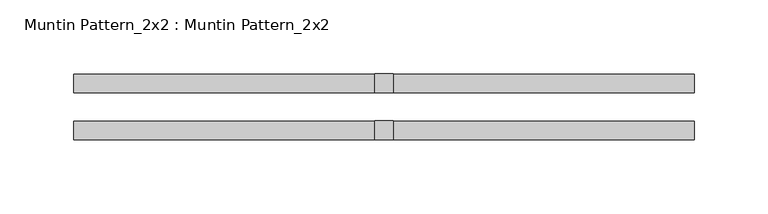
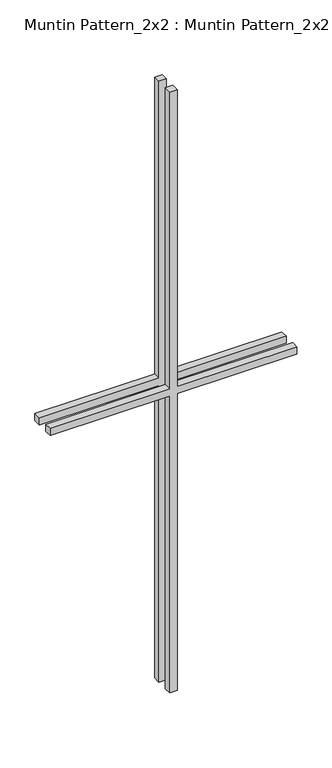
"""IFC4 building model written with IfcOpenShell, lengths in millimetres: proxy geometry, Muntin Pattern_2x2 : Muntin Pattern_2x2."""

from ifc_helpers import new_model, si_unit, frame, origin, place, context, project, spatial, polyline, outline, extrude, source, transform, mapped, element, save


def muntin_pattern_2x2_muntin_pattern_2x2_4aee108e(model_context):
    return source(origin(), model_context, "Body", "SweptSolid", [
        extrude(outline(polyline([(546.1, -6.35), (546.1, -209.55), (533.4, -209.55), (533.4, -6.35), (0.0, -6.35), (0.0, 6.35), (533.4, 6.35), (533.4, 209.55), (546.1, 209.55), (546.1, 6.35), (1079.5, 6.35), (1079.5, -6.35), (546.1, -6.35)])), frame((0.0, 9.525, 0.0), z_axis=(0.0, 1.0, 0.0), x_axis=(0.0, 0.0, 1.0)), (0.0, 0.0, 1.0), 12.7),
        extrude(outline(polyline([(546.1, -6.35), (546.1, -209.55), (533.4, -209.55), (533.4, -6.35), (0.0, -6.35), (0.0, 6.35), (533.4, 6.35), (533.4, 209.55), (546.1, 209.55), (546.1, 6.35), (1079.5, 6.35), (1079.5, -6.35), (546.1, -6.35)])), frame((0.0, -22.225, 0.0), z_axis=(0.0, 1.0, 0.0), x_axis=(0.0, 0.0, 1.0)), (0.0, 0.0, 1.0), 12.7),
    ])


if __name__ == "__main__":
    model = new_model("IFC4")
    model_context = context("Model", 3, world=origin())
    ifc_project = project(units=[si_unit("LENGTHUNIT", "METRE", prefix="MILLI")], contexts=[model_context])
    site = spatial("IfcSite", under=ifc_project)
    building = spatial("IfcBuilding", under=site)
    placement = place(None, origin())
    muntin_pattern_2x2_muntin_pattern_2x2_shape = muntin_pattern_2x2_muntin_pattern_2x2_4aee108e(model_context)
    element("IfcBuildingElementProxy", 1, Name="Muntin Pattern_2x2 : Muntin Pattern_2x2", ObjectType="Muntin Pattern_2x2 : Muntin Pattern_2x2", at=placement, inside=building, context=model_context, shape_type="MappedRepresentation", body=[
        mapped(muntin_pattern_2x2_muntin_pattern_2x2_shape, transform((0.0, 0.0, 0.0), x_axis=(1.0, 0.0, 0.0), y_axis=(0.0, 1.0, 0.0), z_axis=(0.0, 0.0, 1.0))),
    ])
    save(model, "model.ifc")

# Revit data of these elements
# Type "Muntin Pattern_2x2 : Muntin Pattern_2x2"
#   Width [instance default] = 4' - 0"
#   Thickness = 0' - 0 1/2"
#   Height [instance default] = 4' - 0"
#   Distance = 0' - 0 3/4"
#   Interior Material [instance default] = none
#   Exterior Material [instance default] = none
#   Default Elevation = 0
# Element 1 (IfcBuildingElementProxy, "Muntin Pattern_2x2 : Muntin Pattern_2x2")
#   Width = 1' - 4 1/2"
#   Height = 3' - 6 1/2"
#   Interior Material = Wood - Stained
#   Exterior Material = Clad - White
#   Materials on its faces: "Clad - White", "Wood - Stained"
# Materials
#   "Clad - White": class "Wood", colour RGB 242 242 238, transparency 0, Cost = 0
#   "Wood - Stained": class "Wood", colour RGB 224 178 126, transparency 0, Cost = 0
